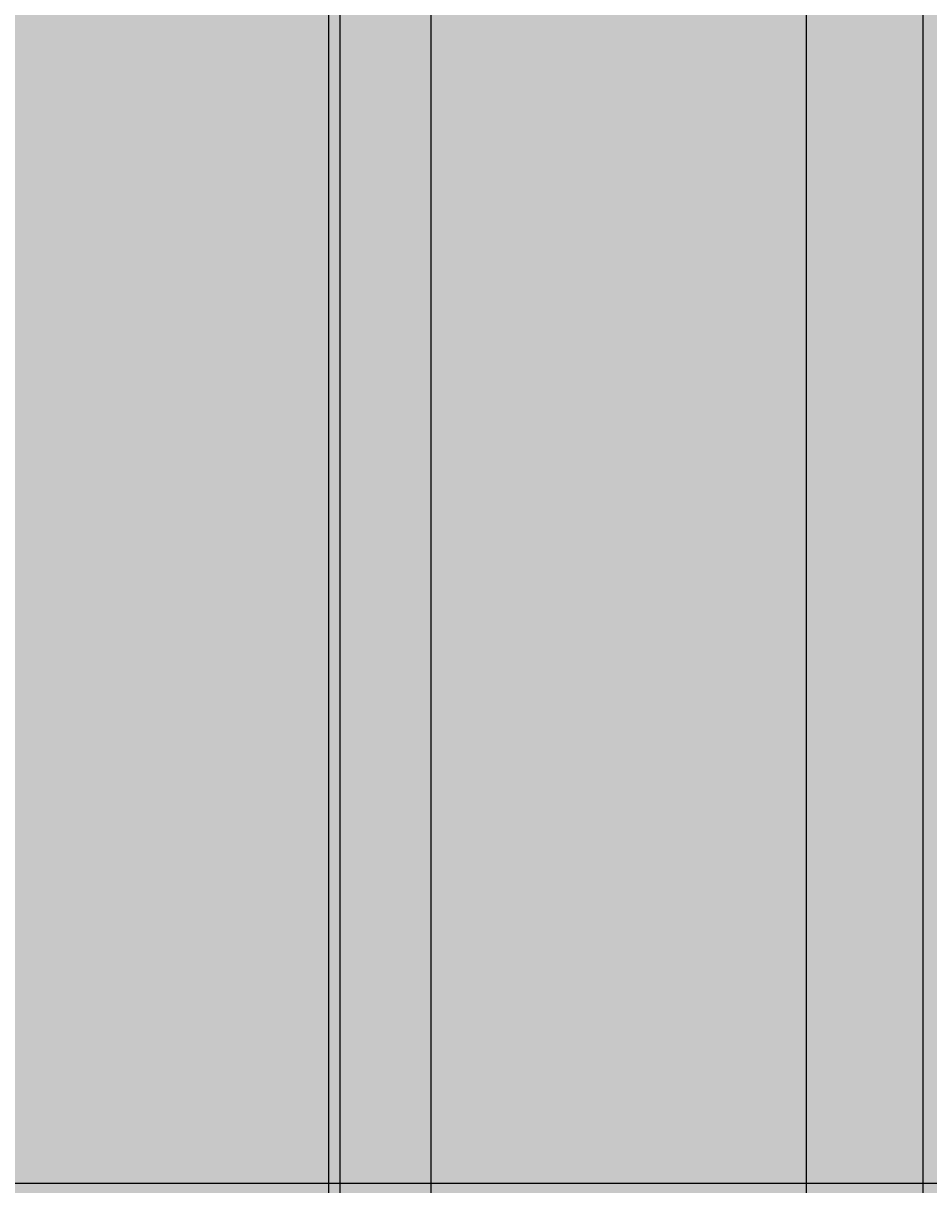
# Model space of a CAD drawing. Units: inches. Extents: x 4508 to 4723, y 847 to 1020.
# Tile 13 of 32: x 4590 to 4631, y 905 to 956. Entities that reach past the tile are written whole.
import ezdxf

# ---------------------------------------------------------------- set-up
doc = ezdxf.new("R2010")
doc.units = ezdxf.units.IN
for name, color, linetype, lineweight in [('A-ANNO-DIMS', 2, 'Continuous', 18), ('A-FURN', 8, 'Continuous', 25), ('A-WALL-PATT', 254, 'Continuous', 13)]:
    doc.layers.add(name, color=color, linetype=linetype, lineweight=lineweight)
doc.styles.get("Standard").update_dxf_attribs({"font": 'arial.ttf'})
doc.dimstyles.get("Standard").update_dxf_attribs({"dimtxt": 0.18, "dimasz": 0.18, "dimexe": 0.18, "dimexo": 0.0625, "dimgap": 0.09, "dimtad": 0, "dimtih": 1, "dimtoh": 1, "dimdec": 4, "dimzin": 0, "dimdsep": 46, "dimtxsty": 'Standard', "dimcen": 0.09, "dimadec": 0, "dimazin": 0, "dimtfac": 1, "dimtdec": 4, "dimtofl": 0, "dimtmove": 0, "dimatfit": 3, "dimfxl": 1, "dimtolj": 1, "dimtzin": 0, "dimarcsym": 0})

# ---------------------------------------------------------------- blocks, each defined once
blk = doc.blocks.new('*D29')
at = {"layer": 'A-ANNO-DIMS', "color": 0, "lineweight": -2, "transparency": 16777216}
for p, q in [((4577.994, 903.809), (4577.994, 1002.877)), ((4603.994, 903.809), (4603.994, 1002.877)), ((4578.174, 1002.697), (4590.773, 1002.697)), ((4603.814, 1002.697), (4591.214, 1002.697))]:
    blk.add_line(p, q, dxfattribs=at)
at = {"layer": 'A-ANNO-DIMS', "color": 0, "lineweight": 9, "transparency": 16777216}
for points in [[(4578.174, 1002.727), (4578.174, 1002.667), (4577.994, 1002.697)], [(4603.814, 1002.727), (4603.814, 1002.667), (4603.994, 1002.697)]]:
    blk.add_solid(points, dxfattribs=at)
at = {"layer": 'Defpoints', "color": 0, "lineweight": 9, "transparency": 16777216}
for p in [(4603.994, 1002.697), (4577.994, 903.747), (4603.994, 903.747)]:
    blk.add_point(p, dxfattribs=at)
at = {"layer": 'A-ANNO-DIMS', "color": 0, "transparency": 16777216, "insert": (4590.994, 1002.697), "char_height": 0.18, "attachment_point": 5}
blk.add_mtext('\\A1;26', dxfattribs=at)
blk = doc.blocks.new('*D30')
at = {"layer": 'A-ANNO-DIMS', "color": 0, "lineweight": -2, "transparency": 16777216}
for p, q in [((4604.494, 903.809), (4604.494, 1002.877)), ((4630.494, 903.809), (4630.494, 1002.877)), ((4604.674, 1002.697), (4617.273, 1002.697)), ((4630.314, 1002.697), (4617.714, 1002.697))]:
    blk.add_line(p, q, dxfattribs=at)
at = {"layer": 'A-ANNO-DIMS', "color": 0, "lineweight": 9, "transparency": 16777216}
for points in [[(4604.674, 1002.727), (4604.674, 1002.667), (4604.494, 1002.697)], [(4630.314, 1002.727), (4630.314, 1002.667), (4630.494, 1002.697)]]:
    blk.add_solid(points, dxfattribs=at)
at = {"layer": 'Defpoints', "color": 0, "lineweight": 9, "transparency": 16777216}
for p in [(4630.494, 1002.697), (4604.494, 903.747), (4630.494, 903.747)]:
    blk.add_point(p, dxfattribs=at)
at = {"layer": 'A-ANNO-DIMS', "color": 0, "transparency": 16777216, "insert": (4617.494, 1002.697), "char_height": 0.18, "attachment_point": 5}
blk.add_mtext('\\A1;26', dxfattribs=at)
blk = doc.blocks.new('*D34')
at = {"layer": 'A-ANNO-DIMS', "color": 0, "lineweight": -2, "transparency": 16777216}
for p, q in [((4608.562, 892.49), (4608.562, 1002.877)), ((4625.298, 892.49), (4625.298, 1002.877)), ((4608.742, 1002.697), (4616.475, 1002.697)), ((4625.118, 1002.697), (4617.385, 1002.697))]:
    blk.add_line(p, q, dxfattribs=at)
at = {"layer": 'A-ANNO-DIMS', "color": 0, "lineweight": 9, "transparency": 16777216}
for points in [[(4608.742, 1002.727), (4608.742, 1002.667), (4608.562, 1002.697)], [(4625.118, 1002.727), (4625.118, 1002.667), (4625.298, 1002.697)]]:
    blk.add_solid(points, dxfattribs=at)
at = {"layer": 'Defpoints', "color": 0, "lineweight": 9, "transparency": 16777216}
for p in [(4625.298, 1002.697), (4608.562, 892.428), (4625.298, 892.428)]:
    blk.add_point(p, dxfattribs=at)
at = {"layer": 'A-ANNO-DIMS', "color": 0, "transparency": 16777216, "insert": (4616.93, 1002.697), "char_height": 0.18, "attachment_point": 5}
blk.add_mtext('\\A1;16.737', dxfattribs=at)

msp = doc.modelspace()

# ---------------------------------------------------------------- hatches: boundary and pattern name
at = {"layer": 'A-WALL-PATT', "transparency": 33554508}
h = msp.add_hatch(color=256, dxfattribs=at)
h.dxf.hatch_style = 1
h.paths.add_polyline_path([(4661.6706, 954.043, -0.3739004), (4658.5765, 957.6021, -1), (4665.7646, 957.6021, -0.3739004), (4662.6706, 954.043), (4662.6706, 944.4021, -0.2114781), (4670.3062, 945.0869), (4670.3062, 968.0592, -0.4632086), (4663.3246, 973.9783, -0.4632086), (4670.3062, 979.8975), (4670.3062, 994.7469), (4588.9938, 994.7469), (4588.9938, 904.7469), (4657.9938, 904.7469), (4657.9938, 886.7469), (4549.9938, 886.7469), (4549.9938, 878.7469), (4693.9938, 878.7469), (4693.9938, 994.7469), (4671.8062, 994.7469), (4671.8062, 979.4411, -0.2941682), (4675.3246, 973.9783, -0.2941682), (4671.8062, 968.5156), (4671.8062, 944.4278, -0.2741114), (4676.7298, 936.1217, -0.2741114), (4671.8062, 927.8155), (4671.8062, 907.6998, -0.3779645), (4677.0562, 901.7469, -0.3779645), (4671.8062, 895.7939), (4671.8062, 883.7469), (4670.3062, 883.7469), (4670.3062, 895.7939, -0.3779645), (4665.0562, 901.7469, -0.3779645), (4670.3062, 907.6998), (4670.3062, 927.1564, -0.2114781), (4662.6706, 927.8412), (4662.6706, 918.2003, -0.3739004), (4665.7646, 914.6412, -1), (4658.5765, 914.6412, -0.3739004), (4661.6706, 918.2003), (4661.6706, 928.4807, -0.2391825), (4657.7936, 936.1217, -0.2391825), (4661.6706, 943.7626)])
at = {"layer": 'A-WALL-PATT', "transparency": 33554681}
h = msp.add_hatch(color=256, dxfattribs=at)
h.dxf.hatch_style = 1
h.paths.add_polyline_path([(4577.4938, 903.7469), (4550.9938, 903.7469), (4550.9938, 887.7469), (4577.4938, 887.7469)], flags=0)
h.paths.add_polyline_path([(4603.9938, 903.7469), (4577.9938, 903.7469), (4577.9938, 887.7469), (4603.9938, 887.7469)], flags=0)
h.paths.add_polyline_path([(4656.9938, 903.7469), (4630.9938, 903.7469), (4630.9938, 887.7469), (4656.9938, 887.7469)], flags=0)
h.paths.add_polyline_path([(4657.9938, 904.7469), (4549.9938, 904.7469), (4549.9938, 886.7469), (4657.9938, 886.7469)])
h.paths.add_polyline_path([(4656.9938, 903.7469), (4656.9938, 887.7469), (4550.9938, 887.7469), (4550.9938, 903.7469)], flags=16)

# ---------------------------------------------------------------- linework, layer by layer
at = {"layer": 'A-FURN'}
msp.add_lwpolyline([(4657.9938, 886.7469), (4549.9938, 886.7469), (4549.9938, 904.7469), (4657.9938, 904.7469)], close=True, dxfattribs=at)

# ---------------------------------------------------------------- dimensions: what is measured, and where the dimension line sits
at = {"layer": 'A-ANNO-DIMS'}
for base, p1, p2, override, picture, middle in [((4603.9938, 1002.6969), (4577.9938, 903.7469), (4603.9938, 903.7469), {"dimdec": 0, "dimlfac": 1, "dimrnd": 0, "dimzin": 0, "dimdsep": 46, "dimlunit": 2}, '*D29', (4590.9938, 1002.6969)), ((4630.4938, 1002.6969), (4604.4938, 903.7469), (4630.4938, 903.7469), {"dimdec": 0, "dimlfac": 1, "dimrnd": 0, "dimzin": 0, "dimdsep": 46, "dimlunit": 2}, '*D30', (4617.4938, 1002.6969)), ((4625.2983, 1002.6969), (4608.5617, 892.4277), (4625.2983, 892.4277), {"dimdec": 3, "dimlfac": 1, "dimrnd": 0, "dimzin": 0, "dimdsep": 46, "dimlunit": 2}, '*D34', (4616.93, 1002.6969))]:
    dim = msp.add_linear_dim(base=base, p1=p1, p2=p2, dimstyle='Standard', override=override, dxfattribs=at)
    dim.commit()
    dim.dimension.update_dxf_attribs({"geometry": picture, "text_midpoint": middle})

doc.saveas('drawing.dxf')
